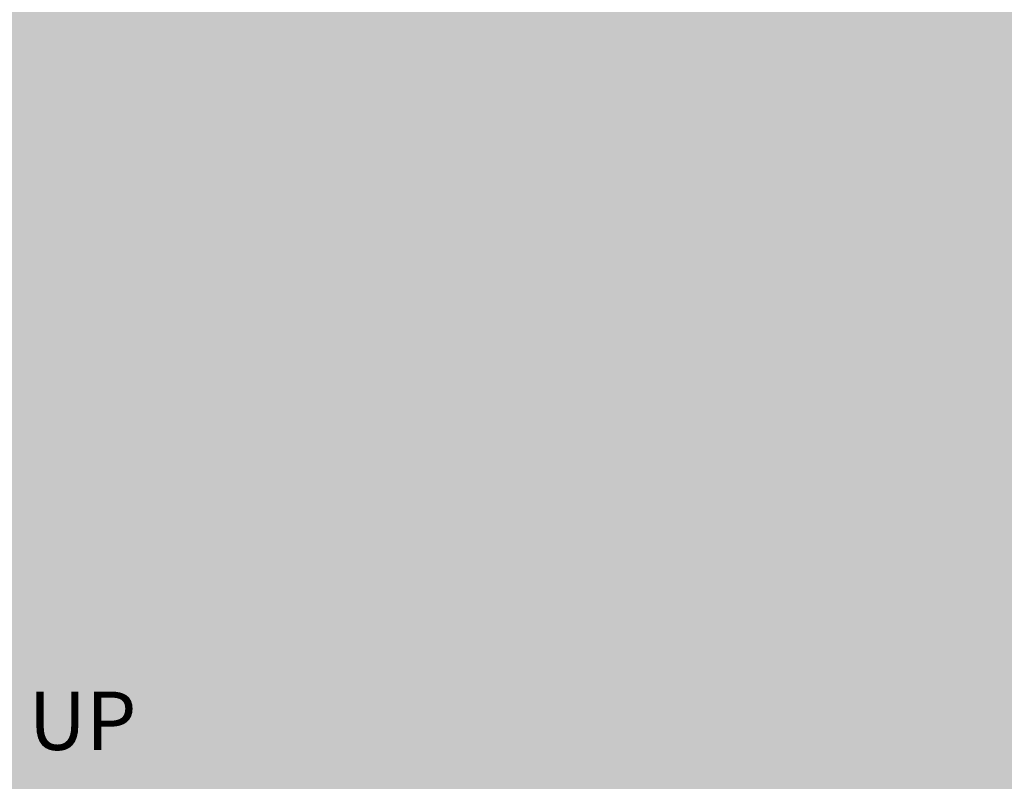
# Model space of a CAD drawing. Units: millimetres. Extents: x -229 to 16545, y -10488 to 4272.
# Tile 9 of 29: x 5862 to 9556, y -4126 to -1268. Entities that reach past the tile are written whole.
import ezdxf

# ---------------------------------------------------------------- set-up
doc = ezdxf.new("R2010")
doc.units = ezdxf.units.MM
doc.layers.add('A-ANNO-SYMB', color=7, linetype='Continuous', lineweight=18)
doc.layers.add('A-FLOR-PATT', color=254, linetype='Continuous', lineweight=13, true_color=0xfeeab9)
doc.styles.get("Standard").update_dxf_attribs({"font": 'arial.ttf'})

msp = doc.modelspace()

# ---------------------------------------------------------------- hatches: boundary and pattern name
at = {"layer": 'A-FLOR-PATT', "transparency": 33554592}
h = msp.add_hatch(color=256, dxfattribs=at)
h.dxf.hatch_style = 1
h.paths.add_polyline_path([(7975.933, -5325.772), (7943.121, -5325.772), (7943.121, -4576.49, 0.40145271), (7225.933, -5325.772, 0.40145271), (6508.746, -4576.49), (6508.746, -5325.772), (6475.933, -5325.772), (6475.933, -5438.272), (5975.933, -5438.272), (5975.933, -7267.724), (5975.933, -7438.272), (6478.619, -7438.272), (6463.448, -7355.919), (6464.88, -7356.837), (6463.849, -7358.097), (6478.619, -7438.272), (6610.327, -7438.272), (6632.656, -7409.564), (6632.525, -7406.967), (6634.208, -7407.569), (6619.273, -7426.77), (6654.466, -7438.272), (7610.517, -7438.272), (7607.41, -7421.409), (7608.842, -7422.327), (7607.812, -7423.587), (7610.517, -7438.272), (7975.933, -7438.272)])
h.paths.add_polyline_path([(13785.933, -1208.272), (9555.933, -1208.272), (9555.933, -961.785), (9705.933, -961.785), (9705.933, -918.035), (10704.976, -918.035, 0.40145271), (9705.933, 38.215), (9555.933, 38.215), (9555.933, 2021.728), (5975.933, 2021.728), (5975.933, 755.492), (5745.933, 755.492), (5745.933, 1427.266), (2918.813, 1427.266), (2918.813, -492.942), (5013.319, -492.942), (5013.319, -978.272), (5745.933, -978.272), (5745.933, -397.513), (5975.933, -397.513), (5975.933, -1208.272), (4560.933, -1208.272), (4560.933, -1265.772), (4448.433, -1265.772), (4448.433, -1298.585), (4445.933, -1298.585), (3699.151, -1298.585, 0.40145271), (4448.433, -2015.772), (4560.933, -2015.772), (4560.933, -2384.177), (5745.933, -2384.177), (5799.402, -2384.177), (5799.402, -4518.272), (5975.933, -4518.272), (5975.933, -5208.272), (6475.933, -5208.272), (6475.933, -4575.772), (6508.746, -4575.772), (6508.746, -4576.49, -0.35647263), (7216.672, -5208.272), (7235.194, -5208.272, -0.35647263), (7943.121, -4576.49), (7943.121, -4575.772), (7975.933, -4575.772), (7975.933, -5208.272), (11176.247, -5208.272), (11159.44, -5191.465), (10520.768, -5191.465), (10520.768, -4888.936), (10571.19, -4888.936), (10571.19, -4872.129), (10772.876, -4872.129), (10772.876, -4888.936), (10789.683, -4888.936), (10789.683, -4872.129), (10991.368, -4872.129), (10991.368, -4888.936), (11041.79, -4888.936), (11041.79, -4872.129), (11058.597, -4872.129, -0.09090909), (11428.354, -4872.129), (11445.162, -4872.129), (11445.162, -4888.936), (11529.197, -4888.936), (11529.197, -5191.465), (11327.512, -5191.465), (11310.704, -5208.272), (13785.933, -5208.272)])
h.paths.add_polyline_path([(11047.216, -1630.944, -1), (11402.816, -1630.944, -1)], flags=16)
h.paths.add_polyline_path([(11148.816, -1630.944), (11225.016, -1554.744), (11301.216, -1630.944), (11225.016, -1707.144)], flags=0)
h.paths.add_polyline_path([(11199.616, -1630.944, -1), (11250.416, -1630.944, -1)], flags=0)
h.paths.add_polyline_path([(11588.751, -2096.259), (11588.751, -1543.254, -0.26666697), (12864.918, -1543.254), (12864.918, -2096.259), (12737.302, -2096.259), (12737.302, -2063.121), (11716.368, -2063.121), (11716.368, -2096.259)], flags=16)
h.paths.add_polyline_path([(12012.696, -2489.42), (12600.997, -2489.42), (12600.997, -3666.022), (12012.696, -3666.022)], flags=16)
h.paths.add_polyline_path([(12176.41, -3599.403), (12174.938, -3609.076), (12173.789, -3618.819), (12173.09, -3628.559), (12172.973, -3638.221), (12173.89, -3652.852), (12175.008, -3657.025), (12172.909, -3643.473), (12173.142, -3624.297), (12175.386, -3605.273)], flags=0)
h.paths.add_polyline_path([(8026.289, -286.944), (7737.703, -287.19), (7734.87, -269.156), (8029.092, -268.905)], flags=16)
h.paths.add_polyline_path([(7733.453, -260.139), (7710.784, -115.865), (7557.191, -115.996), (7556.999, 109.744), (7412.687, 132.166), (7412.433, 429.206), (7556.707, 451.876), (7556.568, 614.769), (7412.256, 637.19), (7412.003, 934.231), (7556.276, 956.9), (7556.084, 1182.639), (7709.677, 1182.77), (7732.099, 1327.082), (8029.14, 1327.335), (8051.808, 1183.062), (8205.401, 1183.192), (8205.594, 957.454), (8349.906, 935.031), (8350.159, 637.99), (8205.885, 615.322), (8206.024, 452.43), (8350.336, 430.006), (8350.59, 132.965), (8206.316, 110.298), (8206.509, -115.442), (8052.916, -115.573), (8030.493, -259.885)], flags=16)
h.paths.add_polyline_path([(12261.416, -3475.554), (12262.632, -3486.776), (12264.032, -3497.007), (12265.554, -3506.365), (12267.136, -3514.968), (12268.719, -3522.935), (12271.304, -3535.59), (12273.606, -3548.078), (12275.271, -3561.064), (12275.93, -3574.938), (12275.325, -3590.3), (12273.425, -3607.964), (12270.795, -3625.658), (12268.066, -3641.063), (12266.318, -3649.679), (12265.456, -3653.626), (12263.984, -3659.846), (12264.032, -3659.566), (12264.342, -3658.241), (12264.807, -3656.37), (12265.456, -3653.626), (12266.318, -3649.679), (12267.409, -3644.302), (12268.668, -3637.664), (12270.019, -3630.037), (12271.384, -3621.695), (12272.69, -3612.908), (12273.857, -3603.948), (12274.81, -3595.088), (12275.47, -3586.601), (12275.782, -3578.689), (12275.757, -3571.292), (12275.423, -3564.275), (12274.816, -3557.512), (12273.964, -3550.872), (12272.896, -3544.224), (12271.645, -3537.439), (12270.24, -3530.385), (12267.543, -3517.181), (12264.612, -3501.247), (12261.849, -3481.059)], flags=0)
h.paths.add_polyline_path([(12332.136, -3408.03), (12333.483, -3416.79), (12335.077, -3424.54), (12336.915, -3431.355), (12338.991, -3437.32), (12341.266, -3442.55), (12343.694, -3447.166), (12346.229, -3451.292), (12348.826, -3455.051), (12351.438, -3458.563), (12357.476, -3466.491), (12363.61, -3476.575), (12368.309, -3489.762), (12369.929, -3503.427), (12369.842, -3516.511), (12368.43, -3530.867), (12365.816, -3545.835), (12362.382, -3559.786), (12360.968, -3564.487), (12363.063, -3557.021), (12364.898, -3549.566), (12366.473, -3542.077), (12367.773, -3534.631), (12368.781, -3527.301), (12369.483, -3520.162), (12369.863, -3513.291), (12369.906, -3506.759), (12369.599, -3500.643), (12368.93, -3494.999), (12367.924, -3489.796), (12366.61, -3484.994), (12365.024, -3480.542), (12363.19, -3476.399), (12361.141, -3472.516), (12358.909, -3468.847), (12356.525, -3465.347), (12354.02, -3461.954), (12351.438, -3458.563), (12345.462, -3450.529), (12339.923, -3439.996), (12335.85, -3428.296), (12332.68, -3412.888)], flags=0)
h.paths.add_polyline_path([(12385.287, -3334.612), (12384.977, -3342.409), (12385.02, -3349.196), (12385.4, -3355.066), (12386.104, -3360.105), (12387.112, -3364.41), (12388.412, -3368.071), (12389.987, -3371.181), (12391.823, -3373.832), (12393.919, -3376.097), (12396.337, -3377.978), (12399.153, -3379.462), (12402.445, -3380.531), (12406.289, -3381.172), (12410.758, -3381.371), (12415.935, -3381.106), (12421.893, -3380.368), (12428.658, -3379.159), (12436.069, -3377.55), (12443.907, -3375.635), (12451.961, -3373.505), (12460.015, -3371.254), (12467.853, -3368.971), (12475.263, -3366.749), (12482.029, -3364.68), (12491.877, -3361.657), (12497.701, -3360.107), (12501.639, -3359.288), (12510.135, -3358.326), (12519.662, -3365.412), (12524.243, -3378.911), (12523.764, -3390.7), (12520.746, -3401.577), (12514.248, -3415.634), (12511.518, -3420.418), (12515.856, -3412.154), (12519.153, -3405.024), (12521.516, -3398.804), (12523.049, -3393.276), (12523.865, -3388.212), (12524.059, -3383.441), (12523.7, -3378.958), (12522.853, -3374.815), (12521.576, -3371.054), (12519.931, -3367.722), (12517.982, -3364.865), (12515.786, -3362.529), (12513.405, -3360.758), (12510.877, -3359.588), (12508.136, -3358.982), (12505.086, -3358.897), (12501.639, -3359.288), (12497.701, -3360.107), (12493.183, -3361.309), (12487.988, -3362.851), (12476.403, -3366.408), (12463.335, -3370.326), (12447.372, -3374.788), (12431.759, -3378.604), (12418.504, -3380.974), (12405.811, -3381.624), (12394.725, -3378.025), (12388.039, -3368.367), (12385.583, -3357.877), (12384.826, -3346.204), (12385.428, -3331.059), (12385.953, -3325.719)], flags=0)
h.paths.add_polyline_path([(7880.016, 1173.969), (7880.373, 1175.495), (7880.433, 1175.851), (7879.484, 1171.818)], flags=0)
h.paths.add_polyline_path([(7802.33, 874.962), (7800.771, 885.032), (7798.932, 893.941), (7796.811, 901.774), (7794.419, 908.63), (7791.798, 914.639), (7789.002, 919.945), (7786.083, 924.686), (7783.093, 929.005), (7780.087, 933.043), (7774.996, 939.717), (7768.406, 949.37), (7762.174, 963.427), (7759.342, 978.002), (7758.629, 991.888), (7759.492, 1007.928), (7761.801, 1025.496), (7765.392, 1044.035), (7766.625, 1049.048), (7764.522, 1039.543), (7762.719, 1030.232), (7761.232, 1021.168), (7760.08, 1012.405), (7759.28, 1003.994), (7758.849, 995.988), (7758.806, 988.44), (7759.167, 981.404), (7759.942, 974.914), (7761.104, 968.936), (7762.617, 963.414), (7764.448, 958.299), (7766.559, 953.535), (7768.918, 949.073), (7771.487, 944.856), (7774.232, 940.835), (7777.115, 936.938), (7782.377, 930.041), (7787.845, 922.139), (7793.348, 911.698), (7798.042, 898.247), (7801.702, 880.527)], flags=0)
h.paths.add_polyline_path([(12519.068, -3228.534), (12519.615, -3236.235), (12520.529, -3242.343), (12521.78, -3247.103), (12523.337, -3250.758), (12525.171, -3253.556), (12527.248, -3255.709), (12529.522, -3257.296), (12531.95, -3258.361), (12534.486, -3258.949), (12537.082, -3259.11), (12539.694, -3258.888), (12542.277, -3258.329), (12544.781, -3257.478), (12547.173, -3256.388), (12549.46, -3255.129), (12550.455, -3254.517), (12555.825, -3251.109), (12557.835, -3249.942), (12565.181, -3246.404), (12574.565, -3253.032), (12576.931, -3265.022), (12576.627, -3277.425), (12575.416, -3290.819), (12574.851, -3295.392), (12575.708, -3287.593), (12576.322, -3280.806), (12576.688, -3274.939), (12576.812, -3269.899), (12576.688, -3265.593), (12576.322, -3261.932), (12575.708, -3258.822), (12574.851, -3256.172), (12573.753, -3253.905), (12572.439, -3252.005), (12570.943, -3250.474), (12569.293, -3249.309), (12567.523, -3248.513), (12565.658, -3248.083), (12563.732, -3248.022), (12561.777, -3248.328), (12559.814, -3248.989), (12557.835, -3249.942), (12555.825, -3251.109), (12553.77, -3252.413), (12551.652, -3253.78), (12549.46, -3255.129), (12543.167, -3258.594), (12532.661, -3259.485), (12524.685, -3253.923), (12520.949, -3245.152), (12519.138, -3233.042)], flags=0)
h.paths.add_polyline_path([(7741.293, 790.501), (7741.641, 799.467), (7741.584, 807.269), (7741.141, 814.015), (7740.329, 819.809), (7739.165, 824.757), (7737.667, 828.966), (7735.853, 832.541), (7733.74, 835.586), (7731.348, 838.188), (7728.71, 840.348), (7725.861, 842.052), (7722.836, 843.28), (7719.671, 844.015), (7716.4, 844.237), (7713.06, 843.932), (7709.684, 843.081), (7706.304, 841.686), (7702.923, 839.834), (7699.543, 837.629), (7696.164, 835.178), (7692.784, 832.585), (7684.718, 826.315), (7675.609, 820.63), (7664.001, 817.274), (7654.105, 821.884), (7647.171, 832.02), (7644.191, 846.522), (7646.321, 860.288), (7647.49, 864.223), (7645.946, 857.865), (7645.046, 852.044), (7644.827, 846.557), (7645.243, 841.404), (7646.221, 836.642), (7647.693, 832.318), (7649.587, 828.489), (7651.832, 825.206), (7654.359, 822.523), (7657.097, 820.49), (7659.984, 819.145), (7662.993, 818.452), (7666.108, 818.357), (7669.311, 818.809), (7672.583, 819.755), (7675.908, 821.139), (7679.268, 822.913), (7682.645, 825.021), (7686.025, 827.401), (7689.404, 829.958), (7692.784, 832.585), (7700.505, 838.509), (7709.871, 843.64), (7721.436, 844.698), (7733.277, 837.617), (7739.571, 825.214), (7741.557, 811.049), (7741.669, 795.575)], flags=0)
h.paths.add_polyline_path([(8377.641, 137.216), (8359.607, 134.382), (8359.356, 428.605), (8377.395, 425.802)], flags=16)
h.paths.add_polyline_path([(7650.715, 668.465), (7650.08, 677.319), (7649.023, 684.34), (7647.579, 689.811), (7645.785, 694.012), (7643.675, 697.228), (7641.286, 699.7), (7638.669, 701.521), (7635.876, 702.744), (7632.96, 703.419), (7629.974, 703.601), (7626.971, 703.344), (7624.004, 702.697), (7621.125, 701.717), (7618.375, 700.462), (7615.749, 699.013), (7614.561, 698.279), (7608.435, 694.382), (7606.125, 693.04), (7598.981, 689.594), (7589.669, 693.773), (7585.26, 702.856), (7584.221, 713.11), (7584.49, 724.584), (7585.863, 739.937), (7586.518, 745.277), (7585.539, 736.31), (7584.841, 728.507), (7584.424, 721.761), (7584.288, 715.966), (7584.433, 711.016), (7584.86, 706.807), (7585.567, 703.231), (7586.556, 700.186), (7587.821, 697.58), (7589.332, 695.397), (7591.053, 693.637), (7592.951, 692.3), (7594.989, 691.385), (7597.132, 690.895), (7599.346, 690.826), (7601.594, 691.18), (7603.851, 691.943), (7606.125, 693.04), (7608.435, 694.382), (7610.797, 695.885), (7613.229, 697.458), (7620.475, 701.929), (7632.001, 704.44), (7643.476, 699.417), (7648.536, 687.571), (7650.63, 673.661)], flags=0)
h.paths.add_polyline_path([(7385.628, 136.37), (7385.382, 424.956), (7403.416, 427.789), (7403.667, 133.567)], flags=16)
h.paths.add_polyline_path([(12993.884, -2257.186), (12959.588, -2257.186), (12959.588, -2125.099), (13531.966, -2125.099, -0.19047621), (13531.966, -3974.321), (12959.588, -3974.321), (12959.588, -3842.233), (12993.884, -3842.233)], flags=16)
h.paths.add_polyline_path([(13413.486, -3313.884), (13413.486, -2785.535), (13562.885, -2785.535, -0.04962821), (13562.885, -3313.884)], flags=0)
h.paths.add_polyline_path([(8377.21, 642.241), (8359.176, 639.407), (8358.925, 933.629), (8376.964, 930.826)], flags=16)
h.paths.add_polyline_path([(13086.058, -1864.83), (13086.058, -1449.84), (13501.048, -1449.84), (13501.048, -1864.83)], flags=16)
h.paths.add_polyline_path([(13305.814, -1862.197), (13302.103, -1859.624), (13298.088, -1857.068), (13293.799, -1854.536), (13289.262, -1852.031), (13284.504, -1849.559), (13279.554, -1847.125), (13274.439, -1844.735), (13269.17, -1842.389), (13263.701, -1840.081), (13257.97, -1837.797), (13251.914, -1835.525), (13245.472, -1833.252), (13238.582, -1830.968), (13231.18, -1828.66), (13223.206, -1826.315), (13209.182, -1822.458), (13204.584, -1821.48), (13217.962, -1824.773), (13235.072, -1829.804), (13248.777, -1834.349), (13260.829, -1838.869), (13274.479, -1844.63), (13289.675, -1852.101), (13302.553, -1859.704)], flags=0)
h.paths.add_polyline_path([(13428.104, -1820.994), (13419.007, -1818.141), (13409.95, -1815.4), (13400.766, -1812.747), (13391.271, -1810.151), (13376.087, -1806.251), (13370.618, -1805.019), (13386.304, -1808.794), (13405.087, -1813.928), (13423.014, -1819.354)], flags=0)
h.paths.add_polyline_path([(7385.197, 641.395), (7384.951, 929.98), (7402.986, 932.814), (7403.236, 638.592)], flags=16)
h.paths.add_polyline_path([(13262.537, -1725.526), (13253.246, -1724.74), (13244.516, -1724.117), (13235.94, -1723.625), (13223.267, -1723.062), (13217.598, -1722.912), (13231.966, -1723.397), (13248.733, -1724.359), (13266.899, -1725.895), (13272.802, -1726.502)], flags=0)
h.paths.add_polyline_path([(13191.893, -1641.137), (13208.675, -1640.506), (13214.057, -1640.258), (13197.763, -1640.936)], flags=0)
h.paths.add_polyline_path([(13097.524, -1608.457), (13114.284, -1609.031), (13120.126, -1609.105), (13103.045, -1608.71)], flags=0)
h.paths.add_polyline_path([(13465.328, -1521.577), (13473.906, -1517.015), (13481.761, -1511.636), (13492.562, -1502.076), (13495.327, -1497.933), (13485.818, -1508.858), (13470.208, -1519.547)], flags=0)
h.paths.add_polyline_path([(13175.015, -1500.891), (13184.046, -1501.807), (13192.721, -1502.52), (13201.114, -1503.034), (13209.273, -1503.351), (13217.244, -1503.476), (13225.078, -1503.41), (13232.821, -1503.16), (13240.524, -1502.728), (13248.233, -1502.117), (13255.993, -1501.322), (13263.825, -1500.293), (13271.746, -1498.974), (13279.775, -1497.305), (13287.928, -1495.229), (13296.222, -1492.688), (13304.675, -1489.622), (13313.304, -1485.975), (13322.089, -1481.727), (13330.859, -1477.028), (13339.408, -1472.063), (13347.526, -1467.02), (13355.006, -1462.087), (13364.86, -1455.202), (13367.224, -1453.299), (13358.544, -1459.754), (13343.348, -1469.775), (13326.143, -1479.767), (13309.023, -1488.045), (13292.249, -1494.129), (13276.009, -1498.264), (13260.299, -1500.88), (13244.401, -1502.51), (13228.945, -1503.378), (13213.316, -1503.508), (13197.047, -1502.876), (13180.088, -1501.481)], flags=0)
h.paths.add_polyline_path([(7733.501, 1336.101), (7736.303, 1354.14), (8024.889, 1354.386), (8027.723, 1336.352)], flags=16)

# ---------------------------------------------------------------- texts
at = {"layer": 'A-ANNO-SYMB'}
msp.add_text('UP', height=219.2126, dxfattribs=at).set_placement((5895.185, -4008.402))

doc.saveas('drawing.dxf')
